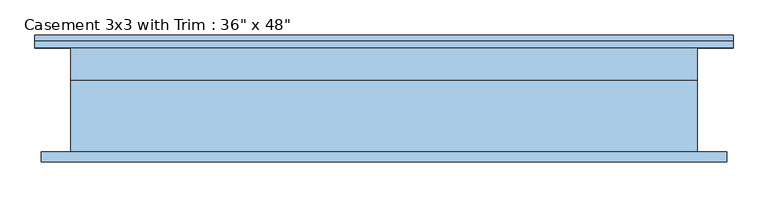
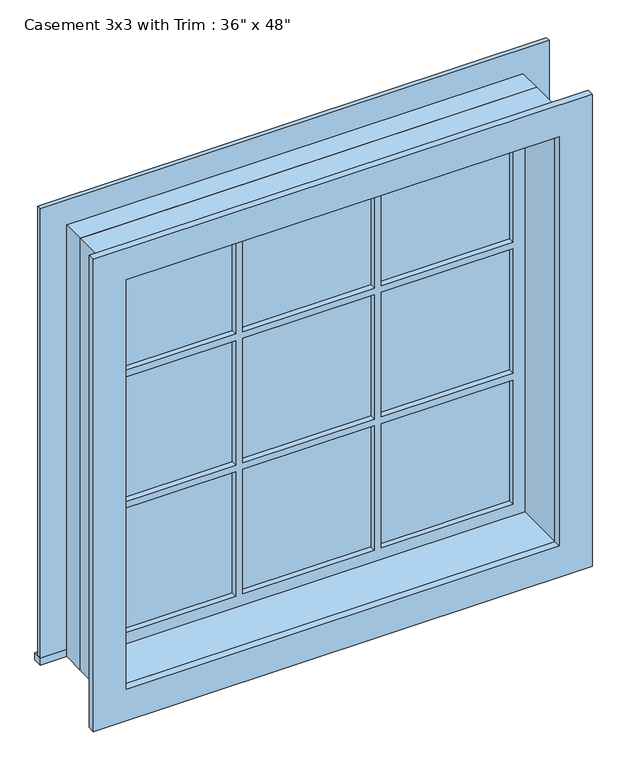
"""IFC4 building model written with IfcOpenShell, lengths in millimetres: window geometry."""

from ifc_helpers import new_model, si_unit, frame, origin, place, context, project, spatial, polyline, outline, extrude, source, transform, mapped, element, save


def window_7418cbd4(model_context):
    return source(origin(), model_context, "Body", "SweptSolid", [
        extrude(outline(polyline([(-679.45, 127.0), (679.45, 127.0), (679.45, 101.6), (-679.45, 101.6), (-679.45, 127.0)])), frame((0.0, 0.0, 914.4), z_axis=(0.0, 0.0, 1.0), x_axis=(1.0, 0.0, 0.0)), (0.0, 0.0, 1.0), 19.05),
        extrude(outline(polyline([(2114.55, -590.55), (2114.55, 590.55), (933.45, 590.55), (933.45, 679.45), (2203.45, 679.45), (2203.45, -679.45), (933.45, -679.45), (933.45, -590.55), (2114.55, -590.55)])), frame((0.0, 101.6, 0.0), z_axis=(0.0, 1.0, 0.0), x_axis=(0.0, 0.0, 1.0)), (0.0, 0.0, 1.0), 12.7),
        extrude(outline(polyline([(194.7333333, 66.675), (546.1, 66.675), (546.1, 53.975), (194.7333333, 53.975), (194.7333333, 66.675)])), frame((0.0, 0.0, 1718.7333333), z_axis=(0.0, 0.0, 1.0), x_axis=(1.0, 0.0, 0.0)), (0.0, 0.0, 1.0), 351.3666667),
        extrude(outline(polyline([(-175.6833333, 66.675), (175.6833333, 66.675), (175.6833333, 53.975), (-175.6833333, 53.975), (-175.6833333, 66.675)])), frame((0.0, 0.0, 1718.7333333), z_axis=(0.0, 0.0, 1.0), x_axis=(1.0, 0.0, 0.0)), (0.0, 0.0, 1.0), 351.3666667),
        extrude(outline(polyline([(-546.1, 66.675), (-194.7333333, 66.675), (-194.7333333, 53.975), (-546.1, 53.975), (-546.1, 66.675)])), frame((0.0, 0.0, 1718.7333333), z_axis=(0.0, 0.0, 1.0), x_axis=(1.0, 0.0, 0.0)), (0.0, 0.0, 1.0), 351.3666667),
        extrude(outline(polyline([(-546.1, 66.675), (-194.7333333, 66.675), (-194.7333333, 53.975), (-546.1, 53.975), (-546.1, 66.675)])), frame((0.0, 0.0, 1348.3166667), z_axis=(0.0, 0.0, 1.0), x_axis=(1.0, 0.0, 0.0)), (0.0, 0.0, 1.0), 351.3666667),
        extrude(outline(polyline([(-175.6833333, 66.675), (175.6833333, 66.675), (175.6833333, 53.975), (-175.6833333, 53.975), (-175.6833333, 66.675)])), frame((0.0, 0.0, 1348.3166667), z_axis=(0.0, 0.0, 1.0), x_axis=(1.0, 0.0, 0.0)), (0.0, 0.0, 1.0), 351.3666667),
        extrude(outline(polyline([(194.7333333, 66.675), (546.1, 66.675), (546.1, 53.975), (194.7333333, 53.975), (194.7333333, 66.675)])), frame((0.0, 0.0, 1348.3166667), z_axis=(0.0, 0.0, 1.0), x_axis=(1.0, 0.0, 0.0)), (0.0, 0.0, 1.0), 351.3666667),
        extrude(outline(polyline([(194.7333333, 66.675), (546.1, 66.675), (546.1, 53.975), (194.7333333, 53.975), (194.7333333, 66.675)])), frame((0.0, 0.0, 977.9), z_axis=(0.0, 0.0, 1.0), x_axis=(1.0, 0.0, 0.0)), (0.0, 0.0, 1.0), 351.3666667),
        extrude(outline(polyline([(-175.6833333, 66.675), (175.6833333, 66.675), (175.6833333, 53.975), (-175.6833333, 53.975), (-175.6833333, 66.675)])), frame((0.0, 0.0, 977.9), z_axis=(0.0, 0.0, 1.0), x_axis=(1.0, 0.0, 0.0)), (0.0, 0.0, 1.0), 351.3666667),
        extrude(outline(polyline([(-546.1, 66.675), (-194.7333333, 66.675), (-194.7333333, 53.975), (-546.1, 53.975), (-546.1, 66.675)])), frame((0.0, 0.0, 977.9), z_axis=(0.0, 0.0, 1.0), x_axis=(1.0, 0.0, 0.0)), (0.0, 0.0, 1.0), 351.3666667),
        extrude(outline(polyline([(2190.75, 666.75), (2190.75, -666.75), (857.25, -666.75), (857.25, 666.75), (2190.75, 666.75)]), holes=[polyline([(2101.85, 577.85), (946.15, 577.85), (946.15, -577.85), (2101.85, -577.85), (2101.85, 577.85)])]), frame((0.0, -120.65, 0.0), z_axis=(0.0, 1.0, 0.0), x_axis=(0.0, 0.0, 1.0)), (0.0, 0.0, 1.0), 19.05),
        extrude(outline(polyline([(2114.55, -590.55), (933.45, -590.55), (933.45, 590.55), (2114.55, 590.55), (2114.55, -590.55)]), holes=[polyline([(2070.1, -194.7333333), (1718.7333333, -194.7333333), (1718.7333333, -546.1), (2070.1, -546.1), (2070.1, -194.7333333)]), polyline([(1699.6833333, -194.7333333), (1348.3166667, -194.7333333), (1348.3166667, -546.1), (1699.6833333, -546.1), (1699.6833333, -194.7333333)]), polyline([(1329.2666667, -194.7333333), (977.9, -194.7333333), (977.9, -546.1), (1329.2666667, -546.1), (1329.2666667, -194.7333333)]), polyline([(2070.1, 175.6833333), (1718.7333333, 175.6833333), (1718.7333333, -175.6833333), (2070.1, -175.6833333), (2070.1, 175.6833333)]), polyline([(1699.6833333, 175.6833333), (1348.3166667, 175.6833333), (1348.3166667, -175.6833333), (1699.6833333, -175.6833333), (1699.6833333, 175.6833333)]), polyline([(1329.2666667, 175.6833333), (977.9, 175.6833333), (977.9, -175.6833333), (1329.2666667, -175.6833333), (1329.2666667, 175.6833333)]), polyline([(2070.1, 546.1), (1718.7333333, 546.1), (1718.7333333, 194.7333333), (2070.1, 194.7333333), (2070.1, 546.1)]), polyline([(1699.6833333, 546.1), (1348.3166667, 546.1), (1348.3166667, 194.7333333), (1699.6833333, 194.7333333), (1699.6833333, 546.1)]), polyline([(1329.2666667, 546.1), (977.9, 546.1), (977.9, 194.7333333), (1329.2666667, 194.7333333), (1329.2666667, 546.1)])]), frame((0.0, 38.1, 0.0), z_axis=(0.0, 1.0, 0.0), x_axis=(0.0, 0.0, 1.0)), (0.0, 0.0, 1.0), 44.45),
        extrude(outline(polyline([(2133.6, -609.6), (914.4, -609.6), (914.4, 609.6), (2133.6, 609.6), (2133.6, -609.6)]), holes=[polyline([(2101.85, -577.85), (2101.85, 577.85), (946.15, 577.85), (946.15, -577.85), (2101.85, -577.85)])]), frame((0.0, -101.6, 0.0), z_axis=(0.0, 1.0, 0.0), x_axis=(0.0, 0.0, 1.0)), (0.0, 0.0, 1.0), 139.7),
        extrude(outline(polyline([(2133.6, 609.6), (2133.6, -609.6), (914.4, -609.6), (914.4, 609.6), (2133.6, 609.6)]), holes=[polyline([(2114.55, 590.55), (933.45, 590.55), (933.45, -590.55), (2114.55, -590.55), (2114.55, 590.55)])]), frame((0.0, 38.1, 0.0), z_axis=(0.0, 1.0, 0.0), x_axis=(0.0, 0.0, 1.0)), (0.0, 0.0, 1.0), 63.5),
    ])


if __name__ == "__main__":
    model = new_model("IFC4")
    model_context = context("Model", 3, world=origin())
    ifc_project = project(units=[si_unit("LENGTHUNIT", "METRE", prefix="MILLI")], contexts=[model_context])
    site = spatial("IfcSite", under=ifc_project)
    building = spatial("IfcBuilding", under=site)
    placement = place(None, origin())
    window_shape = window_7418cbd4(model_context)
    element("IfcWindow", 1, ObjectType="Casement 3x3 with Trim : 36\" x 48\"", at=placement, inside=building, context=model_context, shape_type="MappedRepresentation", body=[
        mapped(window_shape, transform((0.0, 0.0, 0.0), x_axis=(1.0, 0.0, 0.0), y_axis=(0.0, 1.0, 0.0), z_axis=(0.0, 0.0, 1.0))),
    ])
    save(model, "model.ifc")

# Revit data of these elements
# Type "Casement 3x3 with Trim : 36\" x 48\""
#   Type Mark = "10"
#   Construction Type Id = "GSP4R"
#   Assembly Code = "B2020100"
#   Analytic Construction = "1/8 in Pilkington single glazing"
#   Visual Light Transmittance = 0.9
#   Solar Heat Gain Coefficient = 0.78
#   Heat Transfer Coefficient (U) = 0.6496 BTU/(h·ft²·°F)
#   Height = 4' - 0"
#   Default Sill Height = 3' - 0"
#   Trim Projection - Ext. = 0' - 0 1/2"
#   Trim Projection - Int. = 0' - 0 3/4"
#   Trim Width - Exterior = 0' - 3 1/2"
#   Trim Width - Interior = 0' - 3 1/2"
#   Width = 4' - 0"
#   Window Inset = 0' - 0 3/4"
#   Define Thermal Properties by = 1
#   Glass Pane Material = Glass
#   Sash Material = Sash
#   Trim Exterior Material = Trim
#   Trim Interior Material = Trim
#   Wall Closure = (empty or 0)
# Element 1 (IfcWindow, "Casement 3x3 with Trim : 36\" x 48\"")
#   Materials on its faces: "Sash", "Glass", "Trim"
# Materials
#   "Glass": class "Glass", colour RGB 0 128 192, transparency 0.75, Description = "Soda Lime Glass", Cost = 0
#   "Sash": class "Wood", colour RGB 224 178 126, transparency 0
#   "Trim": class "Wood", colour RGB 224 178 126, transparency 0
